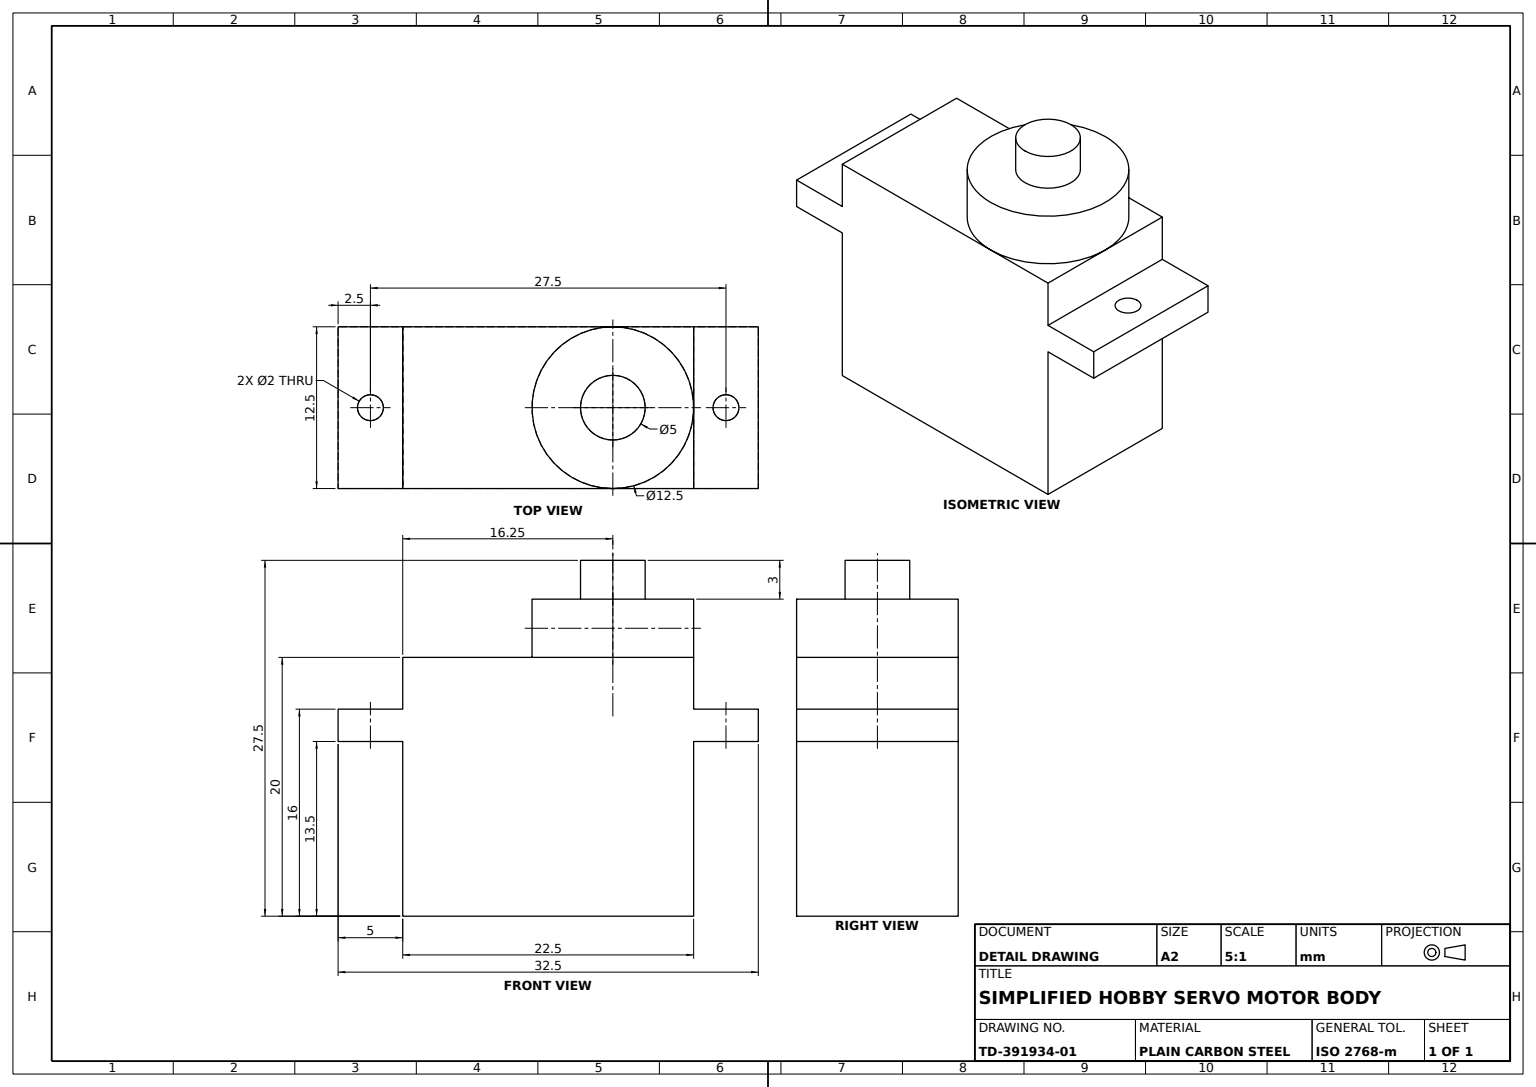
SolidWorks part; units mm, degrees
material "Plain Carbon Steel"
ref_plane "Front Plane" through (0, 0, 0) normal (0, 0, 1) x (1, 0, 0)
ref_plane "Top Plane" through (0, 0, 0) normal (0, 1, 0) x (1, 0, 0)
ref_plane "Right Plane" through (0, 0, 0) normal (1, 0, 0) x (0, 0, -1)
sketch "Servo Case Profile Sketch" plane through (0, 0, 0) normal (0, 0, 1) x (1, 0, 0)
  line L0 (0, 0) -> (0, -4)
  line L1 (0, -4) -> (-5, -4)
  line L2 (-5, -4) -> (-5, -6.5)
  line L3 (-5, -6.5) -> (0, -6.5)
  line L4 (0, -6.5) -> (0, -20)
  line L5 (0, -20) -> (22.5, -20)
  line L6 (22.5, -20) -> (22.5, -6.5)
  line L7 (22.5, -6.5) -> (27.5, -6.5)
  line L8 (27.5, -6.5) -> (27.5, -4)
  line L9 (27.5, -4) -> (22.5, -4)
  line L10 (22.5, -4) -> (22.5, 0)
  line L11 (22.5, 0) -> (0, 0)
  dimension "D1" = 5
  dimension "D2" = 27.5
  dimension "D3" = 13.5
  dimension "D4" = 16
  dimension "D5" = 20
extrude "Servo Case with Mounting Tabs" add sketch "Servo Case Profile Sketch" along normal blind 12.5
sketch "Tab Mounting Hole Sketch" plane through (0, -4, 0) normal (0, 1, 0) x (1, 0, 0)
  line L0 (22.5, -12.5) -> (22.5, 0) construction
  line L1 (27.5, 0) -> (22.5, 0) construction
  circle A0 centre (25, -6.25) radius 1
  circle A1 centre (-2.5, -6.25) radius 1
  dimension "D1" = 2
  dimension "D2" = 2
  dimension "D3" = 2
  dimension "D4" = 2.5
  dimension "D5" = 25
  dimension "D6" = 6.25
extrude "Tab Mounting Hole" cut sketch "Tab Mounting Hole Sketch" against normal blind 2.5
sketch "Output Gear Boss Sketch Ø12.5" plane through (0, 0, 0) normal (0, 1, 0) x (1, 0, 0)
  line L0 (0, -12.5) -> (0, 0) construction
  line L1 (22.5, 0) -> (0, 0) construction
  circle A0 centre (16.25, -6.25) radius 6.25
  dimension "D1" = 12.5
  dimension "D2" = 12.5
  dimension "D3" = 16.25
  dimension "D4" = 6.25
extrude "Output Gear Boss Ø12.5" add sketch "Output Gear Boss Sketch Ø12.5" along normal blind 4.5
sketch "Output Shaft Sketch Ø5" plane through (0, 4.5, 0) normal (0, 1, 0) x (1, 0, 0)
  circle A0 centre (16.25, -6.25) radius 2.5
  dimension "D1" = 5
  dimension "D2" = 5
extrude "Output Shaft Ø5" add sketch "Output Shaft Sketch Ø5" along normal blind 3
